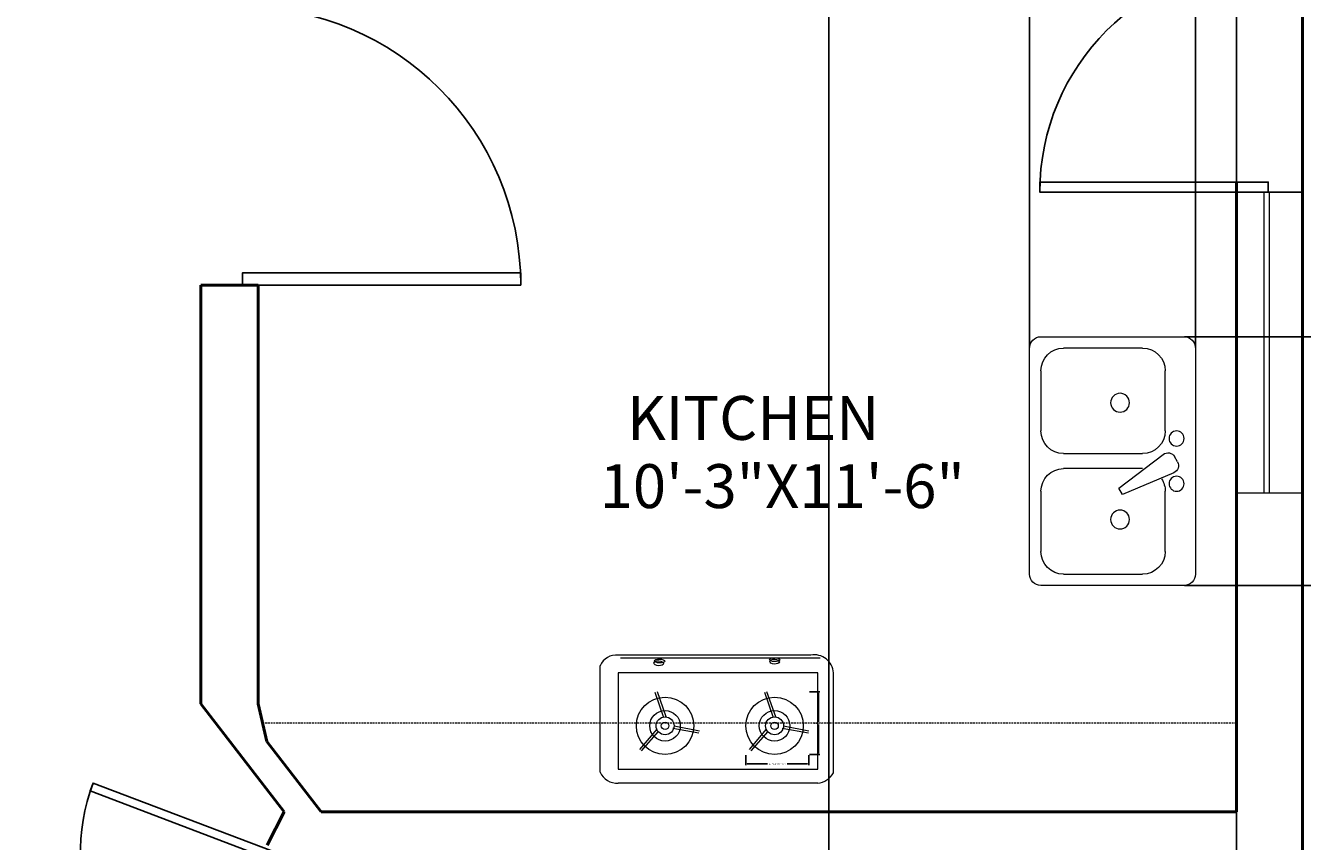
# Model space of a CAD drawing. Units: inches. Extents: x -44 to 461, y -6 to 860.
# Tile 4 of 7: x 185 to 358, y 387 to 498. Entities that reach past the tile are written whole.
import ezdxf

# ---------------------------------------------------------------- set-up
doc = ezdxf.new("R2010")
doc.units = ezdxf.units.IN
doc.header["$MEASUREMENT"] = 0
doc.linetypes.add('HIDDEN', pattern=[0.375, 0.25, -0.125])
for name, color, linetype, lineweight in [('A-ANNO-DIMS', 2, 'Continuous', 18), ('A-AREA-IDEN', 7, 'Continuous', 18), ('A-DOOR', 4, 'Continuous', 25), ('A-EQPM', 8, 'Continuous', 18), ('A-FLOR-CASE-HIDN', 9, 'HIDDEN', 18), ('PLUMBING FIXTURES', 8, 'Continuous', 18), ('walls', 8, 'Continuous', 50), ('windows', 171, 'Continuous', 18)]:
    doc.layers.add(name, color=color, linetype=linetype, lineweight=lineweight)
doc.styles.add('ATT', font='TXT')
doc.styles.get("Standard").update_dxf_attribs({"font": 'arial.ttf'})
doc.dimstyles.get("Standard").update_dxf_attribs({"dimtxt": 0.18, "dimasz": 0.18, "dimexe": 0.18, "dimexo": 0.0625, "dimgap": 0.09, "dimtad": 0, "dimtih": 1, "dimtoh": 1, "dimdec": 4, "dimzin": 0, "dimdsep": 46, "dimtxsty": 'Standard', "dimcen": 0.09, "dimadec": 0, "dimazin": 0, "dimtfac": 1, "dimtdec": 4, "dimtofl": 0, "dimtmove": 0, "dimatfit": 3, "dimfxl": 1, "dimtolj": 1, "dimtzin": 0, "dimarcsym": 0})

# ---------------------------------------------------------------- blocks, each defined once
blk = doc.blocks.new('15PSNK10')
at = {"color": 0, "linetype": 'ByBlock'}
for p, q in [((20.5, 16.5), (1.5, 16.5)), ((0, 15), (0, -15)), ((7, 15), (17.5, 15)), ((22, -15), (22, 15)), ((4, 4), (4, 12)), ((20.5, 12), (20.5, 4)), ((2.37, -0.1), (2.77, 0.6)), ((10.18, -3.57), (4.27, 0.87)), ((17.5, 1), (7, 1)), ((2.88, -1.54), (9.68, -4.43)), ((7.04, -1), (17.5, -1)), ((4, -12), (4, -4)), ((9.68, -4.43), (10.18, -3.57)), ((20.5, -4), (20.5, -12)), ((17.5, -15), (7, -15)), ((1.5, -16.5), (20.5, -16.5))]:
    blk.add_line(p, q, dxfattribs=at)
for centre, radius in [((10, 7.75), 1.25), ((2.5, 3), 1), ((2.5, -3), 1), ((10, -7.75), 1.25)]:
    blk.add_circle(centre, radius, dxfattribs=at)
for centre, radius, start, end in [((1.5, 15), 1.5, 90, 180), ((20.5, 15), 1.5, 0, 90), ((7, 12), 3, 90, 180), ((17.5, 12), 3, 0, 90), ((7, 4), 3, 180, 270), ((17.5, 4), 3, 270, 0), ((3.63, 0.1), 1, 50.5377, 150), ((3.23, -0.6), 1, 150, 249.4623), ((17.5, -4), 3, 0, 90), ((7, -4), 3, 146.607, 180), ((7, -12), 3, 180, 270), ((17.5, -12), 3, 270, 0), ((1.5, -15), 1.5, 180, 270), ((20.5, -15), 1.5, 270, 0)]:
    blk.add_arc(centre, radius, start, end, dxfattribs=at)
at = {"color": 0, "linetype": 'ByBlock', "style": 'ATT'}
for tag, p, flags in [('ITEM', (0, -26), 3), ('ROOM_NUMBER', (0, -35), 1)]:
    blk.add_attdef(tag, p, '', height=6, dxfattribs=dict(at, flags=flags))
blk = doc.blocks.new('*U12')
for p, q in [((0, 0), (0, -6)), ((40, 0), (40, -6))]:
    blk.add_line(p, q)
blk.add_lwpolyline([(0, 0), (0, 40), (1.75, 40), (1.75, 0)], close=True)
blk.add_arc((0, 0), 40, 0, 90)
blk = doc.blocks.new('WIN-41IN-FRAME')
for p, q in [((0, 40.98), (9, 40.98)), ((0, 40.98), (0, 0)), ((3.73, 40.98), (3.73, 0)), ((4.5, 0), (4.5, 40.98)), ((9, 40.98), (9, 0)), ((9, 0), (0, 0))]:
    blk.add_line(p, q)
blk = doc.blocks.new('HOB-GAS-BURNER')
for p, q in [((3.71, 5.12), (2.57, 8.44)), ((4.08, 5.13), (2.86, 8.53)), ((4.96, 3.59), (8.52, 2.94)), ((5.14, 3.91), (8.59, 3.24)), ((2.78, 3.45), (0.44, 0.7)), ((2.97, 3.13), (0.66, 0.49))]:
    blk.add_line(p, q)
for radius in [3.91, 2.08, 1.22, 0.507]:
    blk.add_circle((3.91, 3.91), radius)
blk = doc.blocks.new('*D46')
at = {"layer": 'A-ANNO-DIMS', "color": 0, "lineweight": -2, "transparency": 16777216}
for p, q in [((282.65, 398.81), (282.65, 397.41)), ((291.24, 398.81), (291.24, 397.41)), ((282.83, 397.59), (285.61, 397.59)), ((291.06, 397.59), (288.28, 397.59))]:
    blk.add_line(p, q, dxfattribs=at)
at = {"layer": 'A-ANNO-DIMS', "color": 0, "transparency": 16777216}
for points in [[(282.83, 397.62), (282.83, 397.56), (282.65, 397.59)], [(291.06, 397.62), (291.06, 397.56), (291.24, 397.59)]]:
    blk.add_solid(points, dxfattribs=at)
at = {"layer": 'Defpoints', "color": 0, "transparency": 16777216}
for p in [(282.65, 398.88), (291.24, 398.88), (291.24, 397.59)]:
    blk.add_point(p, dxfattribs=at)
at = {"layer": 'A-ANNO-DIMS', "color": 0, "transparency": 16777216, "insert": (286.95, 397.59), "char_height": 0.18, "attachment_point": 5}
blk.add_mtext('\\A1;BURNER 8.5877 TYP.', dxfattribs=at)
blk = doc.blocks.new('*D47')
at = {"layer": 'A-ANNO-DIMS', "color": 0, "lineweight": -2, "transparency": 16777216}
for p, q in [((291.3, 407.4), (292.71, 407.4)), ((292.53, 407.22), (292.53, 403.32)), ((292.53, 399.06), (292.53, 402.96)), ((291.3, 398.88), (292.71, 398.88))]:
    blk.add_line(p, q, dxfattribs=at)
at = {"layer": 'A-ANNO-DIMS', "color": 0, "transparency": 16777216}
for points in [[(292.5, 407.22), (292.56, 407.22), (292.53, 407.4)], [(292.5, 399.06), (292.56, 399.06), (292.53, 398.88)]]:
    blk.add_solid(points, dxfattribs=at)
at = {"layer": 'Defpoints', "color": 0, "transparency": 16777216}
for p in [(291.24, 407.4), (292.53, 407.4), (291.24, 398.88)]:
    blk.add_point(p, dxfattribs=at)
at = {"layer": 'A-ANNO-DIMS', "color": 0, "transparency": 16777216, "insert": (292.53, 403.14), "char_height": 0.18, "attachment_point": 5}
blk.add_mtext('\\A1;8.5265 TYP.', dxfattribs=at)
blk = doc.blocks.new('*D50')
at = {"layer": 'A-ANNO-DIMS', "color": 0, "lineweight": -2, "transparency": 16777216}
for p, q in [((293.95, 562.12), (293.95, -5.53)), ((349.45, 562.12), (349.45, -5.53)), ((294.13, -5.35), (321.16, -5.35)), ((349.27, -5.35), (322.23, -5.35))]:
    blk.add_line(p, q, dxfattribs=at)
at = {"layer": 'A-ANNO-DIMS', "color": 0, "transparency": 16777216}
for points in [[(294.13, -5.32), (294.13, -5.38), (293.95, -5.35)], [(349.27, -5.32), (349.27, -5.38), (349.45, -5.35)]]:
    blk.add_solid(points, dxfattribs=at)
at = {"layer": 'Defpoints', "color": 0, "transparency": 16777216}
for p in [(293.95, 562.18), (349.45, 562.18), (349.45, -5.35)]:
    blk.add_point(p, dxfattribs=at)
at = {"layer": 'A-ANNO-DIMS', "color": 0, "transparency": 16777216, "insert": (321.7, -5.35), "char_height": 0.18, "attachment_point": 5}
blk.add_mtext('\\A1;55.5000', dxfattribs=at)
blk = doc.blocks.new('*D53')
at = {"layer": 'A-ANNO-DIMS', "color": 0, "lineweight": -2, "transparency": 16777216}
for p, q in [((321.29, 454.3), (321.29, 859.63)), ((321.47, 859.45), (332.05, 859.45)), ((343.69, 859.45), (333.11, 859.45)), ((343.87, 454.3), (343.87, 859.63))]:
    blk.add_line(p, q, dxfattribs=at)
at = {"layer": 'A-ANNO-DIMS', "color": 0, "transparency": 16777216}
for points in [[(321.47, 859.48), (321.47, 859.42), (321.29, 859.45)], [(343.69, 859.48), (343.69, 859.42), (343.87, 859.45)]]:
    blk.add_solid(points, dxfattribs=at)
at = {"layer": 'Defpoints', "color": 0, "transparency": 16777216}
for p in [(343.87, 859.45), (321.29, 454.23), (343.87, 454.23)]:
    blk.add_point(p, dxfattribs=at)
at = {"layer": 'A-ANNO-DIMS', "color": 0, "transparency": 16777216, "insert": (332.58, 859.45), "char_height": 0.18, "attachment_point": 5}
blk.add_mtext('\\A1;22.5824', dxfattribs=at)
blk = doc.blocks.new('*D54')
at = {"layer": 'A-ANNO-DIMS', "color": 0, "lineweight": -2, "transparency": 16777216}
for p, q in [((342.39, 455.77), (461.03, 455.77)), ((460.85, 455.59), (460.85, 439.02)), ((460.85, 422.08), (460.85, 438.65)), ((342.39, 421.9), (461.03, 421.9))]:
    blk.add_line(p, q, dxfattribs=at)
at = {"layer": 'A-ANNO-DIMS', "color": 0, "transparency": 16777216}
for points in [[(460.82, 455.59), (460.88, 455.59), (460.85, 455.77)], [(460.82, 422.08), (460.88, 422.08), (460.85, 421.9)]]:
    blk.add_solid(points, dxfattribs=at)
at = {"layer": 'Defpoints', "color": 0, "transparency": 16777216}
for p in [(342.33, 455.77), (460.85, 455.77), (342.33, 421.9)]:
    blk.add_point(p, dxfattribs=at)
at = {"layer": 'A-ANNO-DIMS', "color": 0, "transparency": 16777216, "insert": (460.85, 438.84), "char_height": 0.18, "attachment_point": 5}
blk.add_mtext('\\A1;33.8736', dxfattribs=at)

msp = doc.modelspace()

# ---------------------------------------------------------------- linework, layer by layer
at = {"layer": 'A-EQPM'}
for p, q in [((291.50749, 412.414), (265.27086, 412.414)), ((262.82382, 396.47233), (262.82382, 411.00778)), ((265.59965, 412.03292), (292.77184, 412.03292)), ((292.44306, 410.02021), (265.27086, 410.02021)), ((265.27086, 410.02021), (265.27086, 396.87979)), ((292.44306, 396.87979), (292.44306, 410.02021)), ((294.5842, 396.39798), (294.5842, 410.02021)), ((265.27086, 396.87979), (292.44306, 396.87979)), ((292.44306, 394.99531), (265.27086, 394.99531))]:
    msp.add_line(p, q, dxfattribs=at)
for centre, radius, start, end in [((265.01694, 410.02364), 2.40381, 83.9363585, 156.8940119), ((291.97527, 409.84111), 2.61507, 3.9270714, 100.3045183), ((265.04615, 397.38859), 2.40381, 202.4061647, 275.3638181), ((292.26396, 397.60424), 2.61507, 273.9270714, 332.5307975)]:
    msp.add_arc(centre, radius, start, end, dxfattribs=at)
for centre, major_axis, ratio in [((270.79, 411.29687), (0.66386, -0.04287), 0.49283971), ((270.89763, 411.61565), (0.71319, -0.0202), 0.376973373), ((286.56763, 411.79293), (0.71319, -0.0202), 0.376973373), ((286.56002, 411.52408), (0.66386, -0.04287), 0.49283971)]:
    msp.add_ellipse(centre, major_axis=major_axis, ratio=ratio, dxfattribs=at)
at = {"layer": 'A-FLOR-CASE-HIDN'}
msp.add_line((216.82434, 403.20944), (349.44568, 403.20944), dxfattribs=at)
at = {"layer": 'walls'}
for p, q in [((358.44568, 752.5501), (358.44568, 262.0501)), ((349.44568, 476.83097), (349.44568, 391.0501)), ((349.44568, 476.83097), (349.44568, 391.0501)), ((208.42435, 447.69249), (208.42435, 462.80268)), ((208.42435, 462.80268), (216.22433, 462.80268)), ((216.22433, 462.80268), (216.22433, 405.76777)), ((208.42435, 447.69249), (208.42435, 405.76777)), ((208.42435, 405.76777), (219.77987, 391.0501)), ((216.22433, 405.76777), (217.42435, 400.65111)), ((217.42435, 400.65111), (224.83208, 391.0501)), ((219.77987, 391.0501), (217.44568, 386.5501)), ((224.83208, 391.0501), (349.44568, 391.0501))]:
    msp.add_line(p, q, dxfattribs=at)

# ---------------------------------------------------------------- block references
at = {"layer": 'A-DOOR'}
for p, xscale, yscale, zscale, rotation in [((353.77957, 475.47002), 0.7776860473082563, 0.7776860473082563, 0.7776860473082563, 90), ((214.10795, 462.80268), -0.9472671488816434, 0.9472671488816434, 0.9472671488816434, 270), ((217.96705, 385.78549), -0.6473174777509669, 0.6473174777509668, 0.6473174777509666, 69.19349462187056)]:
    msp.add_blockref('*U12', p, dxfattribs=dict(at, xscale=xscale, yscale=yscale, zscale=zscale, rotation=rotation))
at = {"layer": 'A-EQPM'}
for p in [(267.739, 398.876), (282.6521, 398.876)]:
    msp.add_blockref('HOB-GAS-BURNER', p, dxfattribs=at)
at = {"layer": 'PLUMBING FIXTURES', "xscale": -1.026473487929304, "yscale": 1.026473487929304, "zscale": 1.026473487929304}
msp.add_blockref('15PSNK10', (343.87134, 438.83588), dxfattribs=at)
at = {"layer": 'windows'}
msp.add_blockref('WIN-41IN-FRAME', (349.446, 434.48519), dxfattribs=at)

# ---------------------------------------------------------------- texts
at = {"layer": 'A-AREA-IDEN'}
for s, height, p in [('KITCHEN', 5.974025, (266.48205, 441.72861)), ('10\'-3"X11\'-6"', 5.9740246, (262.74424, 432.4448))]:
    msp.add_text(s, height=height, dxfattribs=at).set_placement(p)

# ---------------------------------------------------------------- dimensions: what is measured, and where the dimension line sits
at = {"layer": 'A-ANNO-DIMS'}
for base, p1, p2, picture, middle in [((343.87134, 859.4501), (321.28892, 454.23298), (343.87134, 454.23298), '*D53', (332.58013, 859.4501)), ((349.44569, -5.3499), (293.94569, 562.17916), (349.44569, 562.17916), '*D50', (321.69569, -5.3499))]:
    dim = msp.add_linear_dim(base=base, p1=p1, p2=p2, dimstyle='Standard', override={"dimdec": 4, "dimlfac": 1, "dimrnd": 0, "dimzin": 0, "dimdsep": 46, "dimlunit": 2}, dxfattribs=at)
    dim.commit()
    dim.dimension.update_dxf_attribs({"geometry": picture, "text_midpoint": middle})
dim = msp.add_linear_dim(base=(460.84569, 455.77269), p1=(342.33163, 421.89906), p2=(342.33163, 455.77269), angle=90, dimstyle='Standard', override={"dimdec": 4, "dimlfac": 1, "dimrnd": 0, "dimzin": 0, "dimdsep": 46, "dimlunit": 2}, dxfattribs=at)
dim.commit()
dim.dimension.update_dxf_attribs({"geometry": '*D54', "text_midpoint": (460.84569, 438.83588)})
dim = msp.add_linear_dim(base=(292.52748, 407.40271), p1=(291.23933, 398.87622), p2=(291.23933, 407.40271), angle=90, text='<> TYP.', dimstyle='Standard', override={"dimdec": 4, "dimlfac": 1, "dimrnd": 0, "dimzin": 0, "dimdsep": 46, "dimlunit": 2}, dxfattribs=at)
dim.commit()
dim.dimension.update_dxf_attribs({"geometry": '*D47', "text_midpoint": (292.52748, 403.13947)})
dim = msp.add_linear_dim(base=(291.23933, 397.58807), p1=(282.65162, 398.87622), p2=(291.23933, 398.87622), text='BURNER <> TYP.', dimstyle='Standard', override={"dimdec": 4, "dimlfac": 1, "dimrnd": 0, "dimzin": 0, "dimdsep": 46, "dimlunit": 2}, dxfattribs=at)
dim.commit()
dim.dimension.update_dxf_attribs({"geometry": '*D46', "text_midpoint": (286.94547, 397.58807)})

doc.saveas('drawing.dxf')
